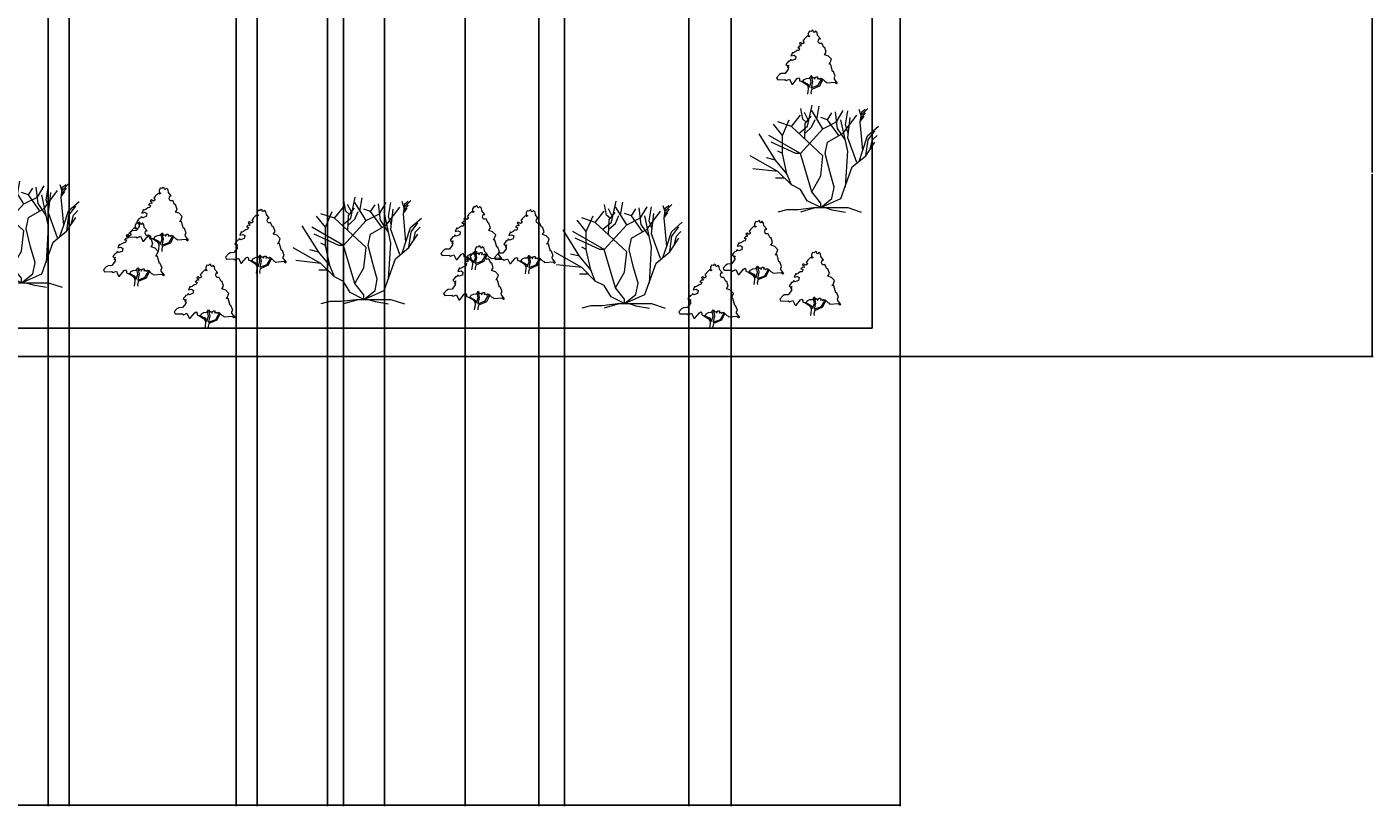
# Model space of a CAD drawing. Units: inches. Extents: x -47 to 496, y -43 to 706.
# Tile 2 of 6: x 209 to 496, y -43 to 123. Entities that reach past the tile are written whole.
import ezdxf

# ---------------------------------------------------------------- set-up
doc = ezdxf.new("R2010")
doc.units = ezdxf.units.IN
for name, color, linetype, lineweight in [('A-ANNO-DIMS', 2, 'Continuous', 18), ('C-PROP', 7, 'Continuous', 25), ('L-PLNT', 3, 'Continuous', 13)]:
    doc.layers.add(name, color=color, linetype=linetype, lineweight=lineweight)
doc.styles.get("Standard").update_dxf_attribs({"font": 'arial.ttf'})
doc.dimstyles.get("Standard").update_dxf_attribs({"dimtxt": 0.18, "dimasz": 0.18, "dimexe": 0.18, "dimexo": 0.0625, "dimgap": 0.09, "dimtad": 0, "dimtih": 1, "dimtoh": 1, "dimdec": 4, "dimzin": 0, "dimdsep": 46, "dimtxsty": 'Standard', "dimcen": 0.09, "dimadec": 0, "dimazin": 0, "dimtfac": 1, "dimtdec": 4, "dimtofl": 0, "dimtmove": 0, "dimatfit": 3, "dimfxl": 1, "dimtolj": 1, "dimtzin": 0, "dimarcsym": 0})

# ---------------------------------------------------------------- blocks, each defined once
blk = doc.blocks.new('*U6')
for p, q in [((-14.88, 18.24), (-12.96, 20.64)), ((-12.471, 19.775), (-12.898, 22.044)), ((-11.28, 19.619), (-12.104, 21.184)), ((-11.921, 18.836), (-10.64, 20.401)), ((-11.433, 18.289), (-10.457, 22.749)), ((-8.16, 17.76), (-10.56, 21.6)), ((-9.48, 19.775), (-8.992, 22.592)), ((-7.2, 19.68), (-8.64, 20.16)), ((-7.2, 19.68), (-6.24, 21.12)), ((-5.086, 17.741), (-5.513, 21.34)), ((-5.28, 19.2), (-3.84, 21.6)), ((-3.84, 16.8), (-0.96, 20.64)), ((-3.377, 18.602), (-2.888, 21.575)), ((-2.88, 15.84), (-2.4, 20.16)), ((-0.508, 21.888), (-0.081, 20.558)), ((-0.203, 19.149), (0.102, 21.34)), ((-0.142, 19.384), (0.59, 20.401)), ((-0.02, 20.01), (0.896, 21.105)), ((0.041, 20.714), (1.384, 22.044)), ((0.102, 21.34), (0.835, 21.888)), ((-16.8, 16.32), (-18.72, 18.72)), ((-14.88, 18.24), (-17.76, 19.2)), ((-16.8, 16.32), (-15.36, 19.68)), ((-8.16, 12), (-14.88, 18.24)), ((-13.325, 16.724), (-11.433, 18.289)), ((-12.96, 12.48), (-8.16, 17.76)), ((-11.677, 19.071), (-12.471, 19.775)), ((-12.043, 15.628), (-11.921, 18.836)), ((-11.982, 16.802), (-10.579, 18.054)), ((-10.579, 18.054), (-9.846, 19.697)), ((-8.16, 17.76), (-5.28, 19.2)), ((-4.8, 16.32), (-7.2, 19.68)), ((-3.377, 15.315), (-5.086, 17.819)), ((-2.88, 12.96), (-4.32, 19.68)), ((-2.766, 16.802), (-3.377, 18.602)), ((0.346, 13.203), (-0.203, 19.149)), ((1.323, 16.254), (3.642, 18.289)), ((1.44, 15.36), (2.88, 17.28)), ((-18.24, 11.04), (-21.755, 16.655)), ((-12.96, 12.48), (-19.68, 16.32)), ((-13.92, 12.48), (-19.2, 14.88)), ((-16.8, 12.48), (-16.8, 16.32)), ((-7.68, 12.48), (-7.2, 14.88)), ((-7.2, 14.88), (-3.84, 16.8)), ((-0.96, 10.56), (-2.88, 15.84)), ((0.346, 13.203), (1.323, 16.254)), ((0.96, 12), (1.44, 15.36)), ((0.96, 12), (2.88, 14.88)), ((1.92, 13.44), (2.4, 15.36)), ((2.4, 15.36), (3.36, 16.32)), ((-17.76, 8.64), (-23.663, 11.961)), ((-18.24, 11.04), (-20.16, 11.52)), ((-16.8, 12.48), (-17.76, 12.96)), ((-15.84, 8.16), (-16.8, 12.48)), ((-12.96, 12.48), (-13.92, 12.48)), ((-10.56, 4.32), (-12.96, 12.48)), ((-8.64, 7.68), (-8.16, 12)), ((-6.72, 8.64), (-7.68, 12.48)), ((-3.36, 5.28), (-2.88, 12.96)), ((-1.92, 9.6), (0.96, 12)), ((-0.48, 10.8), (0.346, 13.203)), ((-17.76, 8.64), (-23.128, 9.222)), ((-15.84, 8.16), (-18.24, 11.04)), ((-14.88, 5.76), (-17.76, 8.64)), ((-5.76, 5.28), (-6.72, 8.64)), ((-4.32, 2.88), (-1.92, 9.6)), ((-16.32, 7.2), (-18.24, 7.2)), ((-14.88, 5.76), (-15.84, 8.16)), ((-12.96, 4.8), (-14.88, 5.76)), ((-10.56, 4.32), (-8.64, 7.68)), ((-11.52, 2.4), (-12.96, 4.8)), ((-8.64, 1.92), (-10.56, 4.32)), ((-8.64, 0.96), (-4.32, 2.88)), ((-8.64, 0.96), (-6.24, 2.88)), ((-6.24, 2.88), (-5.76, 5.28)), ((-15.84, 0.48), (-17.76, 0)), ((-13.44, 0.48), (-15.84, 0.48)), ((-9.6, 0.96), (-13.44, 0.48)), ((-9.6, 0.96), (-12.96, 0)), ((-8.64, 0.96), (-11.52, 2.4)), ((-9.6, 0.96), (-7.68, 0.96)), ((-8.64, 0.96), (-8.64, 1.92)), ((-8.64, 0.96), (-2.88, 0.96)), ((-7.68, 0.96), (-6.24, 0.48)), ((-6.24, 0.48), (-3.36, 0)), ((-2.88, 0.96), (0, 0))]:
    blk.add_line(p, q)
blk = doc.blocks.new('*U7')
for points in [[(22.0124, 137.721), (18.5475, 141.5624), (15.5282, 138.2446), (13.8028, 139.3505), (13.3714, 142.1153), (11.2148, 143.2214), (8.1954, 140.4564), (4.7447, 141.0094), (2.1567, 136.0326), (2.1567, 131.6088), (5.6074, 129.9499), (3.0193, 128.2909), (0.4313, 130.5029), (-6.9015, 123.3141), (-6.9015, 121.6552), (-9.9208, 119.9963), (-9.0581, 118.3373), (-6.9015, 115.0195), (-10.7835, 112.2546), (-14.6656, 115.0195), (-16.8222, 114.4665), (-17.6849, 112.2546), (-14.6656, 111.7016), (-14.2342, 107.2778), (-17.6065, 107.8307), (-21.5669, 103.9599), (-17.2536, 103.4069), (-18.9789, 97.8771), (-22.8609, 97.3241), (-27.1743, 94.5593), (-32.3504, 91.7944), (-32.7817, 94.0063), (-36.6638, 85.7116), (-29.7624, 87.3705), (-25.449, 84.6056), (-26.743, 77.9699), (-34.507, 75.205), (-37.9578, 77.4169), (-39.2518, 74.099), (-42.2711, 73.5461), (-44.8592, 70.2282), (-47.8786, 66.3574), (-43.9965, 63.0395), (-41.4085, 64.6985), (-44.3346, 59.8898), (-42.2089, 60.1377), (-42.5159, 55.7849), (-49.6039, 46.4502), (-58.2307, 45.8972), (-62.1127, 43.6853), (-68.5828, 36.4966), (-65.9947, 32.0727), (-50.0352, 32.6257), (-47.0159, 30.4138), (-39.6831, 33.7317), (-34.507, 22.6721), (-32.3504, 22.6721), (-22.4296, 34.8376), (-19.4102, 36.4966), (-17.2536, 33.7317), (-17.2536, 29.8608), (-13.8028, 28.7549), (-9.0581, 28.7549), (-7.3328, 32.6257), (-1.7254, 35.3906), (3.8821, 35.9436), (6.4701, 38.1555), (6.9014, 38.7085), (8.1954, 41.4734), (9.9208, 40.3674), (11.2148, 35.9436), (14.2341, 37.6025), (15.0968, 36.4966), (15.9595, 33.7317), (18.9789, 38.7085), (21.9982, 38.7085), (23.2922, 36.4966), (21.9982, 34.2847), (25.4489, 35.3906), (26.743, 33.7317), (29.7623, 35.9436), (32.7817, 34.8376), (38.8204, 28.7549), (41.4084, 27.6489), (43.5651, 25.437), (61.6813, 27.0959), (65.132, 23.7781), (67.7201, 24.884), (60.8186, 33.7317), (60.3873, 37.0495), (62.544, 40.3674), (58.662, 50.874), (56.5053, 50.874), (52.1919, 66.3574), (47.8785, 66.9103), (50.4665, 69.1222), (53.9172, 77.9699), (47.0158, 85.1586), (38.3891, 87.9235), (42.2711, 94.0063)], [(42.2711, 94.0063), (38.8204, 104.5129), (36.6637, 104.5129), (32.3503, 113.9135), (29.7623, 113.3605), (26.743, 113.3605), (24.5862, 117.7844), (25.8802, 123.8671), (29.331, 123.8671), (22.8609, 131.6088), (21.9982, 137.6916)], [(-9.9208, 28.2019), (0, 23.2251), (3.4507, 19.9072), (4.7447, 15.4834), (8.6267, 27.0959), (6.4701, 37.6025)], [(34.5071, 33.1787), (27.1743, 18.2483), (9.0581, 10.5066), (7.7641, 3.8708), (8.1954, 0)], [(8.1954, 40.3674), (11.2148, 27.6489), (8.1954, 13.8245), (24.5862, 19.9072), (32.7817, 34.2847)], [(-12.9401, 28.7549), (-2.588, 22.1191), (0.8626, 17.6953), (1.7253, 11.6125), (0, 0)]]:
    blk.add_lwpolyline(points)
blk = doc.blocks.new('*D12')
at = {"layer": 'A-ANNO-DIMS', "color": 0, "lineweight": -2, "transparency": 16777216}
for p, q in [((25.45, 52.91), (25.45, -42.84)), ((395.45, 52.91), (395.45, -42.84)), ((25.63, -42.66), (210.17, -42.66)), ((395.27, -42.66), (210.74, -42.66))]:
    blk.add_line(p, q, dxfattribs=at)
at = {"layer": 'A-ANNO-DIMS', "color": 0, "transparency": 16777216}
for points in [[(25.63, -42.63), (25.63, -42.69), (25.45, -42.66)], [(395.27, -42.63), (395.27, -42.69), (395.45, -42.66)]]:
    blk.add_solid(points, dxfattribs=at)
at = {"layer": 'Defpoints', "color": 0, "transparency": 16777216}
for p in [(25.45, 52.97), (395.45, 52.97), (395.45, -42.66)]:
    blk.add_point(p, dxfattribs=at)
at = {"layer": 'A-ANNO-DIMS', "color": 0, "transparency": 16777216, "insert": (210.45, -42.66), "char_height": 0.18, "attachment_point": 5}
blk.add_mtext('\\A1;370', dxfattribs=at)
blk = doc.blocks.new('*D20')
at = {"layer": 'A-ANNO-DIMS', "color": 0, "lineweight": -2, "transparency": 16777216}
for p, q in [((359.52, 130.97), (496.14, 130.97)), ((495.96, 130.79), (495.96, 92.15)), ((495.96, 53.15), (495.96, 91.79)), ((395.52, 52.97), (496.14, 52.97))]:
    blk.add_line(p, q, dxfattribs=at)
at = {"layer": 'A-ANNO-DIMS', "color": 0, "transparency": 16777216}
for points in [[(495.93, 130.79), (495.99, 130.79), (495.96, 130.97)], [(495.93, 53.15), (495.99, 53.15), (495.96, 52.97)]]:
    blk.add_solid(points, dxfattribs=at)
at = {"layer": 'Defpoints', "color": 0, "transparency": 16777216}
for p in [(359.45, 130.97), (495.96, 130.97), (395.45, 52.97)]:
    blk.add_point(p, dxfattribs=at)
at = {"layer": 'A-ANNO-DIMS', "color": 0, "transparency": 16777216, "insert": (495.96, 91.97), "char_height": 0.18, "attachment_point": 5}
blk.add_mtext('\\A1;78', dxfattribs=at)
blk = doc.blocks.new('*D21')
at = {"layer": 'A-ANNO-DIMS', "color": 0, "lineweight": -2, "transparency": 16777216}
for p, q in [((213.95, 130.91), (213.95, -42.84)), ((359.45, 130.91), (359.45, -42.84)), ((214.13, -42.66), (286.32, -42.66)), ((359.27, -42.66), (287.09, -42.66))]:
    blk.add_line(p, q, dxfattribs=at)
at = {"layer": 'A-ANNO-DIMS', "color": 0, "transparency": 16777216}
for points in [[(214.13, -42.63), (214.13, -42.69), (213.95, -42.66)], [(359.27, -42.63), (359.27, -42.69), (359.45, -42.66)]]:
    blk.add_solid(points, dxfattribs=at)
at = {"layer": 'Defpoints', "color": 0, "transparency": 16777216}
for p in [(213.95, 130.97), (359.45, 130.97), (359.45, -42.66)]:
    blk.add_point(p, dxfattribs=at)
at = {"layer": 'A-ANNO-DIMS', "color": 0, "transparency": 16777216, "insert": (286.7, -42.66), "char_height": 0.18, "attachment_point": 5}
blk.add_mtext('\\A1;145.5', dxfattribs=at)
blk = doc.blocks.new('*D30')
at = {"layer": 'A-ANNO-DIMS', "color": 0, "lineweight": -2, "transparency": 16777216}
for p, q in [((285.61, 151.6), (285.61, -42.84)), ((213.95, 130.91), (213.95, -42.84)), ((214.13, -42.66), (249.39, -42.66)), ((285.43, -42.66), (250.18, -42.66))]:
    blk.add_line(p, q, dxfattribs=at)
at = {"layer": 'A-ANNO-DIMS', "color": 0, "transparency": 16777216}
for points in [[(214.13, -42.63), (214.13, -42.69), (213.95, -42.66)], [(285.43, -42.63), (285.43, -42.69), (285.61, -42.66)]]:
    blk.add_solid(points, dxfattribs=at)
at = {"layer": 'Defpoints', "color": 0, "transparency": 16777216}
for p in [(285.61, 151.67), (213.95, 130.97), (285.61, -42.66)]:
    blk.add_point(p, dxfattribs=at)
at = {"layer": 'A-ANNO-DIMS', "color": 0, "transparency": 16777216, "insert": (249.78, -42.66), "char_height": 0.18, "attachment_point": 5}
blk.add_mtext('\\A1;71.65', dxfattribs=at)
blk = doc.blocks.new('*D35')
at = {"layer": 'A-ANNO-DIMS', "color": 0, "lineweight": -2, "transparency": 16777216}
for p, q in [((218.45, 484.91), (218.45, -42.84)), ((350.45, 480.41), (350.45, -42.84)), ((218.63, -42.66), (284.18, -42.66)), ((350.27, -42.66), (284.73, -42.66))]:
    blk.add_line(p, q, dxfattribs=at)
at = {"layer": 'A-ANNO-DIMS', "color": 0, "transparency": 16777216}
for points in [[(218.63, -42.63), (218.63, -42.69), (218.45, -42.66)], [(350.27, -42.63), (350.27, -42.69), (350.45, -42.66)]]:
    blk.add_solid(points, dxfattribs=at)
at = {"layer": 'Defpoints', "color": 0, "transparency": 16777216}
for p in [(218.45, 484.97), (350.45, 480.47), (350.45, -42.66)]:
    blk.add_point(p, dxfattribs=at)
at = {"layer": 'A-ANNO-DIMS', "color": 0, "transparency": 16777216, "insert": (284.45, -42.66), "char_height": 0.18, "attachment_point": 5}
blk.add_mtext('\\A1;132', dxfattribs=at)
blk = doc.blocks.new('*D51')
at = {"layer": 'A-ANNO-DIMS', "color": 0, "lineweight": -2, "transparency": 16777216}
for p, q in [((218.45, 621.91), (218.45, -42.84)), ((258.46, 619.91), (258.46, -42.84)), ((218.63, -42.66), (238.08, -42.66)), ((258.28, -42.66), (238.84, -42.66))]:
    blk.add_line(p, q, dxfattribs=at)
at = {"layer": 'A-ANNO-DIMS', "color": 0, "transparency": 16777216}
for points in [[(218.63, -42.63), (218.63, -42.69), (218.45, -42.66)], [(258.28, -42.63), (258.28, -42.69), (258.46, -42.66)]]:
    blk.add_solid(points, dxfattribs=at)
at = {"layer": 'Defpoints', "color": 0, "transparency": 16777216}
for p in [(218.45, 621.97), (258.46, 619.97), (258.46, -42.66)]:
    blk.add_point(p, dxfattribs=at)
at = {"layer": 'A-ANNO-DIMS', "color": 0, "transparency": 16777216, "insert": (238.46, -42.66), "char_height": 0.18, "attachment_point": 5}
blk.add_mtext('\\A1;40.01', dxfattribs=at)
blk = doc.blocks.new('*D54')
at = {"layer": 'A-ANNO-DIMS', "color": 0, "lineweight": -2, "transparency": 16777216}
for p, q in [((273.48, 348.41), (273.48, -42.84)), ((350.45, 348.41), (350.45, -42.84)), ((273.66, -42.66), (311.57, -42.66)), ((350.27, -42.66), (312.36, -42.66))]:
    blk.add_line(p, q, dxfattribs=at)
at = {"layer": 'A-ANNO-DIMS', "color": 0, "transparency": 16777216}
for points in [[(273.66, -42.63), (273.66, -42.69), (273.48, -42.66)], [(350.27, -42.63), (350.27, -42.69), (350.45, -42.66)]]:
    blk.add_solid(points, dxfattribs=at)
at = {"layer": 'Defpoints', "color": 0, "transparency": 16777216}
for p in [(273.48, 348.47), (350.45, 348.47), (350.45, -42.66)]:
    blk.add_point(p, dxfattribs=at)
at = {"layer": 'A-ANNO-DIMS', "color": 0, "transparency": 16777216, "insert": (311.97, -42.66), "char_height": 0.18, "attachment_point": 5}
blk.add_mtext('\\A1;76.97', dxfattribs=at)
blk = doc.blocks.new('*D59')
at = {"layer": 'A-ANNO-DIMS', "color": 0, "lineweight": -2, "transparency": 16777216}
for p, q in [((318.48, 390.41), (318.48, -42.84)), ((350.45, 390.41), (350.45, -42.84)), ((318.66, -42.66), (334, -42.66)), ((350.27, -42.66), (334.93, -42.66))]:
    blk.add_line(p, q, dxfattribs=at)
at = {"layer": 'A-ANNO-DIMS', "color": 0, "transparency": 16777216}
for points in [[(318.66, -42.63), (318.66, -42.69), (318.48, -42.66)], [(350.27, -42.63), (350.27, -42.69), (350.45, -42.66)]]:
    blk.add_solid(points, dxfattribs=at)
at = {"layer": 'Defpoints', "color": 0, "transparency": 16777216}
for p in [(318.48, 390.47), (350.45, 390.47), (350.45, -42.66)]:
    blk.add_point(p, dxfattribs=at)
at = {"layer": 'A-ANNO-DIMS', "color": 0, "transparency": 16777216, "insert": (334.47, -42.66), "char_height": 0.18, "attachment_point": 5}
blk.add_mtext('\\A1;31.975', dxfattribs=at)
blk = doc.blocks.new('*D64')
at = {"layer": 'A-ANNO-DIMS', "color": 0, "lineweight": -2, "transparency": 16777216}
for p, q in [((158.02, 343.91), (158.02, -42.84)), ((218.45, 343.91), (218.45, -42.84)), ((158.2, -42.66), (187.84, -42.66)), ((218.27, -42.66), (188.63, -42.66))]:
    blk.add_line(p, q, dxfattribs=at)
at = {"layer": 'A-ANNO-DIMS', "color": 0, "transparency": 16777216}
for points in [[(158.2, -42.63), (158.2, -42.69), (158.02, -42.66)], [(218.27, -42.63), (218.27, -42.69), (218.45, -42.66)]]:
    blk.add_solid(points, dxfattribs=at)
at = {"layer": 'Defpoints', "color": 0, "transparency": 16777216}
for p in [(158.02, 343.97), (218.45, 343.97), (218.45, -42.66)]:
    blk.add_point(p, dxfattribs=at)
at = {"layer": 'A-ANNO-DIMS', "color": 0, "transparency": 16777216, "insert": (188.24, -42.66), "char_height": 0.18, "attachment_point": 5}
blk.add_mtext('\\A1;60.43', dxfattribs=at)
blk = doc.blocks.new('*D65')
at = {"layer": 'A-ANNO-DIMS', "color": 0, "lineweight": -2, "transparency": 16777216}
for p, q in [((218.45, 348.41), (218.45, -42.84)), ((273.48, 348.41), (273.48, -42.84)), ((218.63, -42.66), (245.57, -42.66)), ((273.3, -42.66), (246.36, -42.66))]:
    blk.add_line(p, q, dxfattribs=at)
at = {"layer": 'A-ANNO-DIMS', "color": 0, "transparency": 16777216}
for points in [[(218.63, -42.63), (218.63, -42.69), (218.45, -42.66)], [(273.3, -42.63), (273.3, -42.69), (273.48, -42.66)]]:
    blk.add_solid(points, dxfattribs=at)
at = {"layer": 'Defpoints', "color": 0, "transparency": 16777216}
for p in [(218.45, 348.47), (273.48, 348.47), (273.48, -42.66)]:
    blk.add_point(p, dxfattribs=at)
at = {"layer": 'A-ANNO-DIMS', "color": 0, "transparency": 16777216, "insert": (245.97, -42.66), "char_height": 0.18, "attachment_point": 5}
blk.add_mtext('\\A1;55.03', dxfattribs=at)
blk = doc.blocks.new('*D73')
at = {"layer": 'A-ANNO-DIMS', "color": 0, "lineweight": -2, "transparency": 16777216}
for p, q in [((213.95, 211.91), (213.95, -42.84)), ((195.95, 202.91), (195.95, -42.84)), ((196.13, -42.66), (204.74, -42.66)), ((213.77, -42.66), (205.17, -42.66))]:
    blk.add_line(p, q, dxfattribs=at)
at = {"layer": 'A-ANNO-DIMS', "color": 0, "transparency": 16777216}
for points in [[(196.13, -42.63), (196.13, -42.69), (195.95, -42.66)], [(213.77, -42.63), (213.77, -42.69), (213.95, -42.66)]]:
    blk.add_solid(points, dxfattribs=at)
at = {"layer": 'Defpoints', "color": 0, "transparency": 16777216}
for p in [(213.95, 211.97), (195.95, 202.97), (213.95, -42.66)]:
    blk.add_point(p, dxfattribs=at)
at = {"layer": 'A-ANNO-DIMS', "color": 0, "transparency": 16777216, "insert": (204.95, -42.66), "char_height": 0.18, "attachment_point": 5}
blk.add_mtext('\\A1;18', dxfattribs=at)
blk = doc.blocks.new('*D74')
at = {"layer": 'A-ANNO-DIMS', "color": 0, "lineweight": -2, "transparency": 16777216}
for p, q in [((213.95, 211.91), (213.95, -42.84)), ((254, 211.91), (254, -42.84)), ((214.13, -42.66), (233.58, -42.66)), ((253.82, -42.66), (234.38, -42.66))]:
    blk.add_line(p, q, dxfattribs=at)
at = {"layer": 'A-ANNO-DIMS', "color": 0, "transparency": 16777216}
for points in [[(214.13, -42.63), (214.13, -42.69), (213.95, -42.66)], [(253.82, -42.63), (253.82, -42.69), (254, -42.66)]]:
    blk.add_solid(points, dxfattribs=at)
at = {"layer": 'Defpoints', "color": 0, "transparency": 16777216}
for p in [(213.95, 211.97), (254, 211.97), (254, -42.66)]:
    blk.add_point(p, dxfattribs=at)
at = {"layer": 'A-ANNO-DIMS', "color": 0, "transparency": 16777216, "insert": (233.98, -42.66), "char_height": 0.18, "attachment_point": 5}
blk.add_mtext('\\A1;40.05', dxfattribs=at)
blk = doc.blocks.new('*D75')
at = {"layer": 'A-ANNO-DIMS', "color": 0, "lineweight": -2, "transparency": 16777216}
for p, q in [((254, 202.91), (254, -42.84)), ((323.91, 202.91), (323.91, -42.84)), ((254.18, -42.66), (288.58, -42.66)), ((323.73, -42.66), (289.33, -42.66))]:
    blk.add_line(p, q, dxfattribs=at)
at = {"layer": 'A-ANNO-DIMS', "color": 0, "transparency": 16777216}
for points in [[(254.18, -42.63), (254.18, -42.69), (254, -42.66)], [(323.73, -42.63), (323.73, -42.69), (323.91, -42.66)]]:
    blk.add_solid(points, dxfattribs=at)
at = {"layer": 'Defpoints', "color": 0, "transparency": 16777216}
for p in [(254, 202.97), (323.91, 202.97), (323.91, -42.66)]:
    blk.add_point(p, dxfattribs=at)
at = {"layer": 'A-ANNO-DIMS', "color": 0, "transparency": 16777216, "insert": (288.96, -42.66), "char_height": 0.18, "attachment_point": 5}
blk.add_mtext('\\A1;69.91', dxfattribs=at)
blk = doc.blocks.new('*D84')
at = {"layer": 'A-ANNO-DIMS', "color": 0, "lineweight": -2, "transparency": 16777216}
for p, q in [((276.84, 266.72), (276.84, -42.84)), ((302.79, 266.72), (302.79, -42.84)), ((277.02, -42.66), (289.42, -42.66)), ((302.61, -42.66), (290.21, -42.66))]:
    blk.add_line(p, q, dxfattribs=at)
at = {"layer": 'A-ANNO-DIMS', "color": 0, "transparency": 16777216}
for points in [[(277.02, -42.63), (277.02, -42.69), (276.84, -42.66)], [(302.61, -42.63), (302.61, -42.69), (302.79, -42.66)]]:
    blk.add_solid(points, dxfattribs=at)
at = {"layer": 'Defpoints', "color": 0, "transparency": 16777216}
for p in [(276.84, 266.78), (302.79, 266.78), (302.79, -42.66)]:
    blk.add_point(p, dxfattribs=at)
at = {"layer": 'A-ANNO-DIMS', "color": 0, "transparency": 16777216, "insert": (289.82, -42.66), "char_height": 0.18, "attachment_point": 5}
blk.add_mtext('\\A1;25.95', dxfattribs=at)

msp = doc.modelspace()

# ---------------------------------------------------------------- linework, layer by layer
at = {"layer": 'C-PROP'}
for p, q in [((395.4545, 671.4711), (395.4545, 52.9711)), ((389.4545, 665.4711), (389.4545, 58.9711)), ((31.4545, 58.9711), (389.4545, 58.9711)), ((70.4545, 58.9711), (389.4545, 58.9711)), ((25.4545, 52.9711), (395.4545, 52.9711))]:
    msp.add_line(p, q, dxfattribs=at)

# ---------------------------------------------------------------- block references
at = {"layer": 'L-PLNT', "xscale": 0.0952451950507636, "yscale": 0.0952451950507636, "zscale": 0.0952451950507636}
for p in [(375.6545, 108.8596), (237.4118, 75.3629), (258.2672, 70.6691), (304.1619, 71.4376), (315.5643, 70.5834), (232.2765, 67.9366), (364.2297, 68.2794), (304.7321, 62.8964), (376.3309, 61.7031), (247.3237, 58.9711), (354.7979, 58.9711)]:
    msp.add_blockref('*U7', p, dxfattribs=at)
at = {"layer": 'L-PLNT'}
for p in [(387.1412, 83.7446), (216.9589, 67.7147), (289.8357, 64.1638), (345.3784, 63.2738)]:
    msp.add_blockref('*U6', p, dxfattribs=at)

# ---------------------------------------------------------------- dimensions: what is measured, and where the dimension line sits
at = {"layer": 'A-ANNO-DIMS'}
for base, p1, p2, override, picture, middle in [((258.4633, -42.6632), (218.4545, 621.9711), (258.4633, 619.9711), {"dimdec": 2, "dimlfac": 1, "dimrnd": 0, "dimzin": 0, "dimdsep": 46, "dimlunit": 2}, '*D51', (238.4589, -42.6632)), ((350.4545, -42.6632), (218.4545, 484.9711), (350.4545, 480.4711), {"dimdec": 0, "dimlfac": 1, "dimrnd": 0, "dimzin": 0, "dimdsep": 46, "dimlunit": 2}, '*D35', (284.4545, -42.6632)), ((350.4545, -42.6632), (318.4798, 390.4711), (350.4545, 390.4711), {"dimdec": 3, "dimlfac": 1, "dimrnd": 0, "dimzin": 0, "dimdsep": 46, "dimlunit": 2}, '*D59', (334.4671, -42.6632)), ((273.4798, -42.6632), (218.4545, 348.4711), (273.4798, 348.4711), {"dimdec": 2, "dimlfac": 1, "dimrnd": 0, "dimzin": 0, "dimdsep": 46, "dimlunit": 2}, '*D65', (245.9671, -42.6632)), ((350.4545, -42.6632), (273.4798, 348.4711), (350.4545, 348.4711), {"dimdec": 2, "dimlfac": 1, "dimrnd": 0, "dimzin": 0, "dimdsep": 46, "dimlunit": 2}, '*D54', (311.9671, -42.6632)), ((218.4545, -42.6632), (158.0229, 343.9711), (218.4545, 343.9711), {"dimdec": 2, "dimlfac": 1, "dimrnd": 0, "dimzin": 0, "dimdsep": 46, "dimlunit": 2}, '*D64', (188.2387, -42.6632)), ((302.7925, -42.6632), (276.8411, 266.7848), (302.7925, 266.7848), {"dimdec": 2, "dimlfac": 1, "dimrnd": 0, "dimzin": 0, "dimdsep": 46, "dimlunit": 2}, '*D84', (289.8168, -42.6632)), ((213.9545, -42.6632), (195.9545, 202.9711), (213.9545, 211.9711), {"dimdec": 0, "dimlfac": 1, "dimrnd": 0, "dimzin": 0, "dimdsep": 46, "dimlunit": 2}, '*D73', (204.9545, -42.6632)), ((254.0024, -42.6632), (213.9545, 211.9711), (254.0024, 211.9711), {"dimdec": 2, "dimlfac": 1, "dimrnd": 0, "dimzin": 0, "dimdsep": 46, "dimlunit": 2}, '*D74', (233.9785, -42.6632)), ((323.9122, -42.6632), (254.0024, 202.9711), (323.9122, 202.9711), {"dimdec": 2, "dimlfac": 1, "dimrnd": 0, "dimzin": 0, "dimdsep": 46, "dimlunit": 2}, '*D75', (288.9573, -42.6632)), ((285.6085, -42.6632), (213.9545, 130.9711), (285.6085, 151.6661), {"dimdec": 2, "dimlfac": 1, "dimrnd": 0, "dimzin": 0, "dimdsep": 46, "dimlunit": 2}, '*D30', (249.7815, -42.6632)), ((359.4545, -42.6632), (213.9545, 130.9711), (359.4545, 130.9711), {"dimdec": 1, "dimlfac": 1, "dimrnd": 0, "dimzin": 0, "dimdsep": 46, "dimlunit": 2}, '*D21', (286.7045, -42.6632)), ((395.4545, -42.6632), (25.4545, 52.9711), (395.4545, 52.9711), {"dimdec": 0, "dimlfac": 1, "dimrnd": 0, "dimzin": 0, "dimdsep": 46, "dimlunit": 2}, '*D12', (210.4545, -42.6632))]:
    dim = msp.add_linear_dim(base=base, p1=p1, p2=p2, dimstyle='Standard', override=override, dxfattribs=at)
    dim.commit()
    dim.dimension.update_dxf_attribs({"geometry": picture, "text_midpoint": middle})
dim = msp.add_linear_dim(base=(495.9572, 130.9711), p1=(395.4545, 52.9711), p2=(359.4545, 130.9711), angle=90, dimstyle='Standard', override={"dimdec": 0, "dimlfac": 1, "dimrnd": 0, "dimzin": 0, "dimdsep": 46, "dimlunit": 2}, dxfattribs=at)
dim.commit()
dim.dimension.update_dxf_attribs({"geometry": '*D20', "text_midpoint": (495.9572, 91.9711)})

doc.saveas('drawing.dxf')
